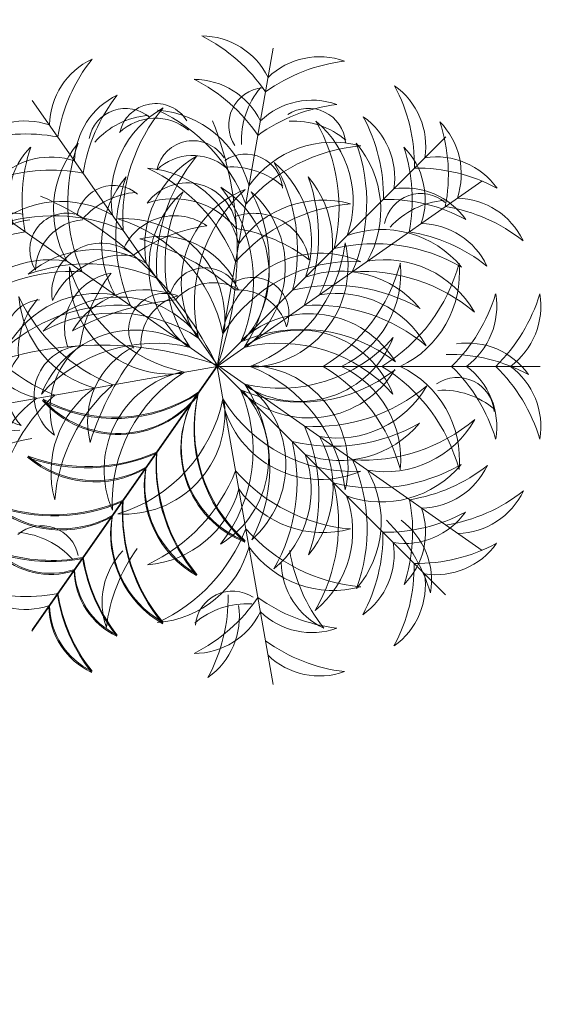
# Model space of a CAD drawing. Units: inches. Extents: x -48 to 50072, y 0 to 21068.
# Tile 26 of 75: x 394 to 415, y 289 to 328. Entities that reach past the tile are written whole.
import ezdxf

# ---------------------------------------------------------------- set-up
doc = ezdxf.new("R2010")
doc.units = ezdxf.units.IN
doc.header["$MEASUREMENT"] = 0
doc.layers.add('A-ANNO-DIMS', color=2, linetype='Continuous', lineweight=18)
doc.layers.add('L-PLNT', color=94, linetype='Continuous', lineweight=13)
doc.styles.get("Standard").update_dxf_attribs({"font": 'arial.ttf'})
doc.dimstyles.get("Standard").update_dxf_attribs({"dimtxt": 8, "dimasz": 0.18, "dimexe": 0.18, "dimexo": 0.0625, "dimgap": 0.09, "dimtad": 0, "dimtih": 1, "dimtoh": 1, "dimdec": 1, "dimzin": 0, "dimdsep": 46, "dimlunit": 4, "dimtxsty": 'Standard', "dimblk": 'ARCHTICK', "dimcen": 0.09, "dimadec": 0, "dimazin": 0, "dimtfac": 1, "dimtdec": 1, "dimtofl": 0, "dimtmove": 0, "dimatfit": 3, "dimldrblk": 'ARCHTICK', "dimfxl": 1, "dimtolj": 1, "dimtzin": 0, "dimarcsym": 0})

# ---------------------------------------------------------------- blocks, each defined once
blk = doc.blocks.new('A$C5D061C3B')
for p, q in [((3.377, 6.679), (3.377, 3.377)), ((1.483, 6.082), (3.377, 3.377)), ((5.259, 6.086), (3.365, 3.381)), ((1.03, 5.716), (3.365, 3.381)), ((5.712, 5.712), (3.377, 3.377)), ((0.125, 3.951), (3.377, 3.377)), ((6.629, 3.951), (3.377, 3.377)), ((0.66, 1.487), (3.365, 3.381)), ((1.483, 0.672), (3.377, 3.377)), ((6.07, 1.487), (3.365, 3.381)), ((3.951, 0.125), (3.377, 3.377)), ((6.082, 1.483), (3.377, 3.377))]:
    blk.add_line(p, q)
for centre, radius, start, end in [((2.763, 5.924), 0.762, 36.29, 99.6243), ((2.145, 5.032), 1.715, 44.0763, 73.3794), ((3.991, 5.924), 0.762, 80.3757, 143.71), ((4.61, 5.032), 1.715, 106.6206, 135.9237), ((3.901, 5.939), 0.762, 125.3757, 188.71), ((4.969, 5.745), 1.715, 151.6206, 180.9237), ((2.419, 5.816), 0.762, 115.3757, 178.71), ((3.438, 5.44), 1.715, 141.6206, 170.9237), ((3.305, 5.444), 1.715, 9.0763, 38.3794), ((4.323, 5.82), 0.762, 1.29, 64.6243), ((1.998, 5.617), 0.762, 125.3757, 188.71), ((3.066, 5.423), 1.715, 151.6206, 180.9237), ((2.763, 5.474), 0.762, 36.29, 99.6243), ((2.145, 4.581), 1.715, 44.0763, 73.3794), ((3.991, 5.474), 0.762, 80.3757, 143.71), ((4.61, 4.581), 1.715, 106.6206, 135.9237), ((3.871, 5.832), 0.38, 94.742, 213.7475), ((4.447, 5.681), 0.826, 139.618, 183.2106), ((4.064, 5.451), 0.762, 1.29, 64.6243), ((3.046, 5.075), 1.715, 9.0763, 38.3794), ((4.744, 5.613), 0.762, 351.29, 54.6243), ((3.676, 5.419), 1.715, 359.0763, 28.3794), ((2.678, 5.447), 0.762, 115.3757, 178.71), ((3.696, 5.07), 1.715, 141.6206, 170.9237), ((3.344, 5.089), 1.056, 119.6063, 189.7511), ((4.177, 4.869), 1.77, 139.9634, 183.6288), ((3.398, 5.094), 1.056, 350.2489, 60.3937), ((2.565, 4.873), 1.77, 356.3712, 40.0366), ((1.413, 5.111), 0.762, 71.29, 134.6243), ((2.317, 5.298), 0.762, 125.3757, 188.71), ((3.385, 5.104), 1.715, 151.6206, 180.9237), ((3.035, 5.062), 1.056, 129.6063, 199.7511), ((3.894, 4.989), 1.77, 149.9634, 193.6288), ((2.422, 4.799), 1.056, 25.2489, 95.3937), ((1.866, 4.14), 1.77, 31.3712, 75.0366), ((4.332, 4.799), 1.056, 84.6063, 154.7511), ((4.888, 4.14), 1.77, 104.9634, 148.6288), ((2.848, 4.985), 1.77, 346.3712, 30.0366), ((3.707, 5.058), 1.056, 340.2489, 50.3937), ((3.357, 5.1), 1.715, 359.0763, 28.3794), ((4.425, 5.294), 0.762, 351.29, 54.6243), ((1.419, 4.026), 1.715, 79.0763, 108.3794), ((1.991, 5.462), 0.38, 139.742, 258.7475), ((2.505, 5.763), 0.826, 184.618, 228.2106), ((5.564, 4.807), 0.762, 80.3757, 143.71), ((6.182, 3.914), 1.715, 106.6206, 135.9237), ((1.13, 4.748), 0.762, 81.29, 144.6243), ((1.671, 4.742), 0.762, 71.29, 134.6243), ((3.46, 4.637), 1.056, 129.6063, 199.7511), ((4.319, 4.565), 1.77, 149.9634, 193.6288), ((3.688, 4.597), 1.056, 119.6063, 189.7511), ((4.522, 4.377), 1.77, 139.9634, 183.6288), ((2.221, 4.381), 1.77, 356.3712, 40.0366), ((3.054, 4.602), 1.056, 350.2489, 60.3937), ((3.283, 4.633), 1.056, 340.2489, 50.3937), ((2.424, 4.56), 1.77, 346.3712, 30.0366), ((5.071, 4.746), 0.762, 45.3757, 108.71), ((5.613, 4.744), 0.762, 35.3757, 98.71), ((1.324, 3.68), 1.715, 89.0763, 118.3794), ((1.677, 3.657), 1.715, 79.0763, 108.3794), ((5.065, 3.661), 1.715, 71.6206, 100.9237), ((5.419, 3.676), 1.715, 61.6206, 90.9237), ((2.422, 4.198), 1.056, 25.2489, 95.3937), ((1.866, 3.54), 1.77, 31.3712, 75.0366), ((4.332, 4.198), 1.056, 84.6063, 154.7511), ((4.888, 3.54), 1.77, 104.9634, 148.6288), ((1.448, 4.43), 0.762, 81.29, 144.6243), ((3.868, 4.321), 1.029, 121.3654, 221.5741), ((4.556, 4.237), 1.557, 141.8122, 203.3335), ((4.035, 4.215), 1.029, 111.3654, 211.5741), ((2.707, 4.219), 1.029, 328.4259, 68.6346), ((2.044, 4.017), 1.557, 346.6665, 48.1878), ((4.698, 4.013), 1.557, 131.8122, 193.3335), ((2.187, 4.233), 1.557, 336.6665, 38.1878), ((2.875, 4.316), 1.029, 318.4259, 58.6346), ((5.294, 4.425), 0.762, 35.3757, 98.71), ((1.642, 3.362), 1.715, 89.0763, 118.3794), ((1.78, 3.994), 1.056, 60.2489, 130.3937), ((4.963, 3.998), 1.056, 49.6063, 119.7511), ((5.1, 3.357), 1.715, 61.6206, 90.9237), ((2.143, 4.564), 1.056, 164.6063, 234.7511), ((1.702, 3.136), 1.77, 66.3712, 110.0366), ((2.888, 4.998), 1.77, 184.9634, 228.6288), ((3.25, 4.435), 1.029, 156.3654, 256.5741), ((3.862, 4.761), 1.557, 176.8122, 238.3335), ((2.893, 4.761), 1.557, 301.6665, 3.1878), ((3.504, 4.435), 1.029, 283.4259, 23.6346), ((5.04, 3.14), 1.77, 69.9634, 113.6288), ((3.866, 4.998), 1.77, 311.3712, 355.0366), ((4.611, 4.564), 1.056, 305.2489, 15.3937), ((1.685, 3.712), 1.056, 70.2489, 140.3937), ((2.734, 4.46), 1.056, 164.6063, 234.7511), ((3.48, 4.893), 1.77, 184.9634, 228.6288), ((3.275, 4.893), 1.77, 311.3712, 355.0366), ((4.02, 4.46), 1.056, 305.2489, 15.3937), ((5.058, 3.707), 1.056, 39.6063, 109.7511), ((0.975, 4.424), 0.762, 160.3757, 223.71), ((1.962, 4.878), 1.715, 186.6206, 215.9237), ((1.12, 4.31), 0.38, 94.742, 213.7475), ((1.696, 4.159), 0.826, 139.618, 183.2106), ((2.358, 3.686), 1.029, 3.4259, 103.6346), ((1.93, 3.14), 1.557, 21.6665, 83.1878), ((4.397, 3.686), 1.029, 76.3654, 176.5741), ((4.824, 3.14), 1.557, 96.8122, 158.3335), ((4.793, 4.878), 1.715, 324.0763, 353.3794), ((5.779, 4.424), 0.762, 316.29, 19.6243), ((1.419, 4.346), 0.762, 160.3757, 223.71), ((2.405, 4.8), 1.715, 186.6206, 215.9237), ((1.757, 2.853), 1.77, 76.3712, 120.0366), ((2.124, 3.502), 1.056, 60.2489, 130.3937), ((4.618, 3.506), 1.056, 49.6063, 119.7511), ((4.985, 2.848), 1.77, 59.9634, 103.6288), ((4.349, 4.8), 1.715, 324.0763, 353.3794), ((5.335, 4.346), 0.762, 316.29, 19.6243), ((4.988, 5.812), 1.715, 279.0763, 308.3794), ((5.365, 4.794), 0.762, 271.29, 334.6243), ((2.109, 3.287), 1.056, 70.2489, 140.3937), ((2.046, 2.644), 1.77, 66.3712, 110.0366), ((4.696, 2.648), 1.77, 69.9634, 113.6288), ((4.633, 3.283), 1.056, 39.6063, 109.7511), ((2.387, 3.752), 0.574, 99.9865, 199.4034), ((3.599, 3.314), 1.651, 142.5759, 170.8942), ((2.182, 2.428), 1.77, 76.3712, 120.0366), ((4.56, 2.424), 1.77, 59.9634, 103.6288), ((1.588, 3.666), 0.38, 94.742, 213.7475), ((2.165, 3.515), 0.826, 139.618, 183.2106), ((2.365, 3.045), 1.029, 38.4259, 138.6346), ((2.84, 3.739), 0.372, 69.2257, 210.1279), ((3.109, 3.59), 0.515, 105.4398, 183.6694), ((4.377, 3.05), 1.029, 41.3654, 141.5741), ((0.762, 3.214), 0.762, 116.29, 179.6243), ((1.534, 2.451), 1.715, 124.0763, 153.3794), ((0.91, 3.875), 0.38, 184.742, 303.7475), ((2.426, 2.879), 1.029, 48.4259, 148.6346), ((2.328, 2.353), 1.557, 56.6665, 118.1878), ((4.414, 2.358), 1.557, 61.8122, 123.3335), ((4.316, 2.875), 1.029, 31.3654, 131.5741), ((1.206, 3.136), 0.762, 116.29, 179.6243), ((1.977, 2.373), 1.715, 124.0763, 153.3794), ((1.062, 4.452), 0.826, 229.618, 273.2106), ((2.51, 2.191), 1.557, 66.6665, 128.1878), ((4.233, 2.187), 1.557, 51.8122, 113.3335), ((6.053, 3.533), 0.38, 146.2525, 265.258), ((4.777, 2.373), 1.715, 26.6206, 55.9237), ((6.629, 3.684), 0.826, 176.7894, 220.382), ((5.549, 3.136), 0.762, 0.3757, 63.71), ((1.811, 2.684), 1.056, 105.2489, 175.3937), ((2.363, 2.022), 1.77, 111.3712, 155.0366), ((2.729, 4.702), 1.557, 221.8122, 283.3335), ((2.527, 4.039), 1.029, 201.3654, 301.5741), ((4.001, 4.702), 1.557, 256.6665, 318.1878), ((4.013, 4.698), 1.557, 256.6665, 318.1878), ((4.203, 4.039), 1.029, 238.4259, 338.6346), ((4.215, 4.035), 1.029, 238.4259, 338.6346), ((4.391, 2.022), 1.77, 24.9634, 68.6288), ((4.943, 2.684), 1.056, 4.6063, 74.7511), ((2.185, 0.015), 3.567, 70.4772, 111.6585), ((2.403, 2.58), 1.056, 105.2489, 175.3937), ((2.955, 1.917), 1.77, 111.3712, 155.0366), ((2.007, 3.071), 0.506, 93.8744, 233.9763), ((2.489, 2.932), 0.825, 128.7536, 199.097), ((2.903, 2.8), 0.855, 116.4477, 194.3672), ((4.744, 1.779), 2.789, 140.4007, 163.139), ((2.741, 3.253), 0.372, 114.2257, 255.1279), ((3.037, 3.338), 0.515, 150.4398, 228.6694), ((3.799, 1.917), 1.77, 24.9634, 68.6288), ((4.352, 2.58), 1.056, 4.6063, 74.7511), ((5.935, 2.842), 0.762, 35.3757, 98.71), ((1.447, 3.129), 0.376, 122.0577, 257.8533), ((1.751, 3.126), 0.529, 140.1845, 223.654), ((2.896, 2.427), 1.029, 83.4259, 183.6346), ((3.359, 1.911), 1.557, 101.6665, 163.1878), ((3.395, 1.911), 1.557, 16.8122, 78.3335), ((3.858, 2.427), 1.029, 356.3654, 96.5741), ((5.741, 1.774), 1.715, 61.6206, 90.9237), ((4.912, 0.157), 3.567, 115.4772, 156.6585), ((6.727, 2.189), 3.567, 160.4772, 201.6585), ((2.412, 2.943), 0.574, 144.9865, 244.4034), ((3.578, 3.49), 1.651, 187.5759, 215.8942), ((2.145, 3.693), 1.056, 209.6063, 279.7511), ((2.365, 4.526), 1.77, 229.9634, 273.6288), ((3.697, 2.369), 1.029, 128.4259, 228.6346), ((4.389, 2.332), 1.557, 146.6665, 208.1878), ((2.341, 2.332), 1.557, 331.8122, 33.3335), ((2.353, 2.328), 1.557, 331.8122, 33.3335), ((3.033, 2.369), 1.029, 311.3654, 51.5741), ((3.045, 2.365), 1.029, 311.3654, 51.5741), ((4.365, 4.526), 1.77, 266.3712, 310.0366), ((4.377, 4.522), 1.77, 266.3712, 310.0366), ((4.585, 3.693), 1.056, 260.2489, 330.3937), ((4.597, 3.688), 1.056, 260.2489, 330.3937), ((1.067, 2.749), 0.376, 122.0577, 257.8533), ((1.37, 2.745), 0.529, 140.1845, 223.654), ((2.328, 4.401), 1.557, 241.8122, 303.3335), ((2.365, 3.709), 1.029, 221.3654, 321.5741), ((1.911, 3.359), 1.557, 286.8122, 348.3335), ((4.035, 2.539), 1.029, 148.4259, 248.6346), ((4.698, 2.741), 1.557, 166.6665, 228.1878), ((4.761, 3.862), 1.557, 211.6665, 273.1878), ((2.427, 2.896), 1.029, 266.3654, 6.5741), ((3.003, 2.844), 0.372, 159.2257, 300.1279), ((3.152, 3.113), 0.515, 195.4398, 273.6694), ((5.474, 3.214), 2.789, 185.4007, 208.139), ((4.435, 3.25), 1.029, 193.4259, 293.6346), ((1.873, 4.181), 1.77, 229.9634, 273.6288), ((1.653, 3.348), 1.056, 209.6063, 279.7511), ((3.45, 2.634), 0.855, 161.4477, 239.3672), ((4.857, 4.181), 1.77, 266.3712, 310.0366), ((4.869, 4.177), 1.77, 266.3712, 310.0366), ((5.077, 3.348), 1.056, 260.2489, 330.3937), ((5.089, 3.344), 1.056, 260.2489, 330.3937), ((4.099, 2.051), 1.77, 156.3712, 200.0366), ((2.632, 2.051), 1.77, 339.9634, 23.6288), ((2.644, 2.046), 1.77, 339.9634, 23.6288), ((1.122, 2.441), 0.38, 139.742, 258.7475), ((1.636, 2.741), 0.826, 184.618, 228.2106), ((3.24, 2.128), 1.056, 150.2489, 220.3937), ((3.49, 2.128), 1.056, 319.6063, 29.7511), ((3.502, 2.124), 1.056, 319.6063, 29.7511), ((1.908, 2.317), 0.38, 139.742, 258.7475), ((2.422, 2.617), 0.826, 184.618, 228.2106), ((2.624, 2.192), 0.506, 138.8744, 278.9763), ((3.064, 2.435), 0.825, 173.7536, 244.097), ((3.942, 2.908), 0.855, 206.4477, 284.3672), ((4.963, 4.749), 2.789, 230.4007, 253.139), ((6.244, 3.948), 1.715, 234.0763, 263.3794), ((2.046, 4.111), 1.77, 249.9634, 293.6288), ((2.124, 3.252), 1.056, 229.6063, 299.7511), ((3.607, 1.706), 1.77, 156.3712, 200.0366), ((4.522, 2.378), 1.77, 176.3712, 220.0366), ((3.124, 1.706), 1.77, 339.9634, 23.6288), ((1.672, 3.7), 1.715, 231.6206, 260.9237), ((1.295, 2.682), 0.762, 205.3757, 268.71), ((3.688, 2.157), 1.056, 170.2489, 240.3937), ((3.136, 1.702), 1.77, 339.9634, 23.6288), ((5.79, 2.962), 0.762, 226.29, 289.6243), ((5.058, 3.7), 1.715, 279.0763, 308.3794), ((5.07, 3.696), 1.715, 279.0763, 308.3794), ((5.435, 2.682), 0.762, 271.29, 334.6243), ((5.447, 2.678), 0.762, 271.29, 334.6243), ((2.748, 1.784), 1.056, 150.2489, 220.3937), ((3.428, 3.603), 1.651, 232.5759, 260.8942), ((2.99, 2.391), 0.574, 189.9865, 289.4034), ((1.917, 2.955), 1.77, 294.9634, 338.6288), ((4.893, 3.48), 1.77, 221.3712, 265.0366), ((3.982, 1.784), 1.056, 319.6063, 29.7511), ((3.994, 1.78), 1.056, 319.6063, 29.7511), ((2.58, 2.403), 1.056, 274.6063, 344.7511), ((4.46, 2.734), 1.056, 215.2489, 285.3937), ((0.926, 2.424), 0.762, 205.3757, 268.71), ((1.303, 3.442), 1.715, 231.6206, 260.9237), ((5.427, 3.442), 1.715, 279.0763, 308.3794), ((5.44, 3.438), 1.715, 279.0763, 308.3794), ((5.804, 2.424), 0.762, 271.29, 334.6243), ((5.816, 2.419), 0.762, 271.29, 334.6243), ((1.702, 3.619), 1.77, 249.9634, 293.6288), ((1.78, 2.76), 1.056, 229.6063, 299.7511), ((2, 1.676), 0.762, 161.29, 224.6243), ((3.086, 1.681), 1.715, 169.0763, 198.3794), ((2.188, 1.837), 0.376, 167.0577, 302.8533), ((2.405, 2.049), 0.529, 185.1845, 268.654), ((4.177, 1.886), 1.77, 176.3712, 220.0366), ((3.81, 2.493), 0.825, 218.7536, 289.097), ((3.671, 2.011), 0.506, 183.8744, 323.9763), ((5.385, 1.584), 0.38, 101.2525, 220.258), ((3.645, 1.681), 1.715, 341.6206, 10.9237), ((4.73, 1.676), 0.762, 315.3757, 18.71), ((3.657, 1.677), 1.715, 341.6206, 10.9237), ((4.742, 1.671), 0.762, 315.3757, 18.71), ((3.344, 1.665), 1.056, 170.2489, 240.3937), ((5.899, 1.283), 0.826, 131.7894, 175.382), ((2.717, 1.423), 1.715, 169.0763, 198.3794), ((2.022, 2.363), 1.77, 294.9634, 338.6288), ((4.998, 2.888), 1.77, 221.3712, 265.0366), ((4.014, 1.423), 1.715, 341.6206, 10.9237), ((1.631, 1.417), 0.762, 161.29, 224.6243), ((5.099, 1.417), 0.762, 315.3757, 18.71), ((3.227, 2.169), 0.826, 229.618, 273.2106), ((3.076, 1.593), 0.38, 184.742, 303.7475), ((2.684, 1.811), 1.056, 274.6063, 344.7511), ((4.564, 2.143), 1.056, 215.2489, 285.3937), ((1.671, 2.012), 0.762, 225.3757, 288.71), ((1.677, 3.098), 1.715, 251.6206, 280.9237), ((2.405, 1.511), 0.529, 185.1845, 268.654), ((3.696, 1.684), 1.715, 189.0763, 218.3794), ((5.808, 1.754), 1.715, 189.0763, 218.3794), ((2.188, 1.299), 0.376, 167.0577, 302.8533), ((3.616, 1.755), 0.529, 230.1845, 313.654), ((3.613, 1.452), 0.376, 212.0577, 347.8533), ((4.79, 1.377), 0.762, 181.29, 244.6243), ((2.678, 1.307), 0.762, 181.29, 244.6243), ((1.419, 2.729), 1.715, 251.6206, 280.9237), ((1.413, 1.643), 0.762, 225.3757, 288.71), ((3.438, 1.315), 1.715, 189.0763, 218.3794), ((2.583, 1.701), 0.826, 229.618, 273.2106), ((2.432, 1.124), 0.38, 184.742, 303.7475), ((2.373, 1.977), 1.715, 296.6206, 325.9237), ((3.528, 0.69), 0.38, 56.2525, 175.258), ((4.8, 2.405), 1.715, 234.0763, 263.3794), ((2.419, 0.938), 0.762, 181.29, 244.6243), ((3.68, 0.113), 0.826, 86.7894, 130.382), ((3.997, 1.374), 0.529, 230.1845, 313.654), ((3.994, 1.071), 0.376, 212.0577, 347.8533), ((3.136, 1.206), 0.762, 270.3757, 333.71), ((4.346, 1.419), 0.762, 226.29, 289.6243), ((2.451, 1.534), 1.715, 296.6206, 325.9237), ((4.878, 1.962), 1.715, 234.0763, 263.3794), ((3.214, 0.762), 0.762, 270.3757, 333.71), ((4.424, 0.975), 0.762, 226.29, 289.6243)]:
    blk.add_arc(centre, radius, start, end)
blk = doc.blocks.new('_ArchTick')
at = {"color": 0, "linetype": 'ByBlock', "const_width": 0.15}
blk.add_lwpolyline([(-0.5, -0.5), (0.5, 0.5)], dxfattribs=at)
blk = doc.blocks.new('*D118')
at = {"layer": 'A-ANNO-DIMS', "color": 0, "lineweight": -2, "transparency": 16777216}
for p, q in [((297.017, 488.712), (297.017, 165.945)), ((463.517, 488.712), (463.517, 165.945)), ((297.017, 166.125), (367.026, 166.125)), ((463.517, 166.125), (393.509, 166.125))]:
    blk.add_line(p, q, dxfattribs=at)
at = {"layer": 'Defpoints', "color": 0, "transparency": 16777216}
for p in [(297.017, 488.775), (463.517, 488.775), (463.517, 166.125)]:
    blk.add_point(p, dxfattribs=at)
at = {"layer": 'A-ANNO-DIMS', "color": 0, "lineweight": -2, "transparency": 16777216, "xscale": 0.18, "yscale": 0.18, "zscale": 0.18, "rotation": 180}
blk.add_blockref('_ArchTick', (297.017, 166.125), dxfattribs=at)
at = {"layer": 'A-ANNO-DIMS', "color": 0, "lineweight": -2, "transparency": 16777216, "xscale": 0.18, "yscale": 0.18, "zscale": 0.18}
blk.add_blockref('_ArchTick', (463.517, 166.125), dxfattribs=at)
at = {"layer": 'A-ANNO-DIMS', "color": 0, "transparency": 16777216, "insert": (380.267, 166.125), "char_height": 8, "attachment_point": 5}
blk.add_mtext('\\A1;166.5', dxfattribs=at)

msp = doc.modelspace()

# ---------------------------------------------------------------- block references
at = {"layer": 'L-PLNT', "xscale": 3.862191520948588, "yscale": 3.862191520948588, "zscale": 3.862191520948588, "rotation": 270}
msp.add_blockref('A$C5D061C3B', (388.535, 326.972), dxfattribs=at)

# ---------------------------------------------------------------- dimensions: what is measured, and where the dimension line sits
at = {"layer": 'A-ANNO-DIMS'}
dim = msp.add_linear_dim(base=(463.517, 166.125), p1=(297.017, 488.775), p2=(463.517, 488.775), dimstyle='Standard', override={"dimdec": 1, "dimlfac": 1, "dimrnd": 0, "dimzin": 0, "dimdsep": 46, "dimlunit": 2}, dxfattribs=at)
dim.commit()
dim.dimension.update_dxf_attribs({"geometry": '*D118', "text_midpoint": (380.267, 166.125)})

doc.saveas('drawing.dxf')
